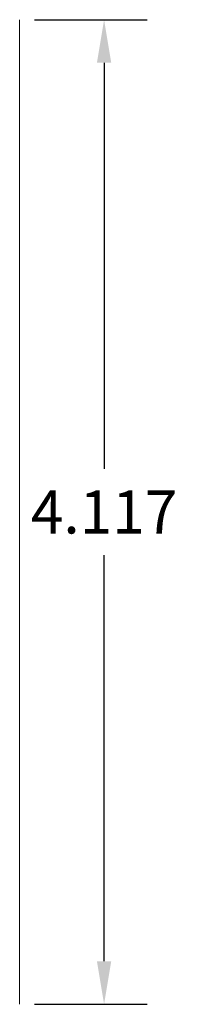
# Model space of a CAD drawing. Units: inches. Extents: x 0 to 0.66, y 7.93 to 12.04.
import ezdxf

# ---------------------------------------------------------------- set-up
doc = ezdxf.new("R2010")
doc.units = ezdxf.units.IN
doc.header["$MEASUREMENT"] = 0
doc.layers.add('M-CONS', color=7, linetype='Continuous', lineweight=18)
doc.layers.add('M-DIMS', color=2, linetype='Continuous', lineweight=18)
doc.styles.get("Standard").update_dxf_attribs({"font": 'arial.ttf'})
doc.dimstyles.get("Standard").update_dxf_attribs({"dimtxt": 0.18, "dimasz": 0.18, "dimexe": 0.18, "dimexo": 0.0625, "dimgap": 0.09, "dimtad": 0, "dimtih": 1, "dimtoh": 1, "dimdec": 4, "dimzin": 0, "dimdsep": 46, "dimtxsty": 'Standard', "dimcen": 0.09, "dimadec": 0, "dimazin": 0, "dimtfac": 1, "dimtdec": 4, "dimtofl": 0, "dimtmove": 0, "dimatfit": 3, "dimfxl": 1, "dimtolj": 1, "dimtzin": 0, "dimarcsym": 0})

# ---------------------------------------------------------------- blocks, each defined once
blk = doc.blocks.new('*D1')
at = {"layer": 'Defpoints', "color": 0, "transparency": 16777216}
for p in [(0, 12.0447), (0.3535, 12.0447), (0, 7.9273)]:
    blk.add_point(p, dxfattribs=at)
at = {"layer": 'M-DIMS', "color": 0, "lineweight": -2, "transparency": 16777216}
for p, q in [((0.0625, 12.0447), (0.5335, 12.0447)), ((0.3535, 11.8647), (0.3535, 10.1664)), ((0.3535, 8.1073), (0.3535, 9.8056)), ((0.0625, 7.9273), (0.5335, 7.9273))]:
    blk.add_line(p, q, dxfattribs=at)
at = {"layer": 'M-DIMS', "color": 0, "transparency": 16777216}
for points in [[(0.3235, 11.8647), (0.3835, 11.8647), (0.3535, 12.0447)], [(0.3235, 8.1073), (0.3835, 8.1073), (0.3535, 7.9273)]]:
    blk.add_solid(points, dxfattribs=at)
at = {"layer": 'M-DIMS', "color": 0, "transparency": 16777216, "insert": (0.3535, 9.986), "char_height": 0.18, "attachment_point": 5}
blk.add_mtext('\\A1;4.117', dxfattribs=at)

msp = doc.modelspace()

# ---------------------------------------------------------------- linework, layer by layer
at = {"layer": 'M-CONS', "extrusion": (-1, 0, 0)}
msp.add_lwpolyline([(-12.0447, 26.6429), (-7.9273, 26.6429), (-7.9273, 22.887), (-12.0447, 22.887)], close=True, dxfattribs=at)

# ---------------------------------------------------------------- dimensions: what is measured, and where the dimension line sits
at = {"layer": 'M-DIMS'}
dim = msp.add_linear_dim(base=(0.3535, 12.0447), p1=(0, 7.9273), p2=(0, 12.0447), angle=90, dimstyle='Standard', override={"dimdec": 3, "dimlfac": 1, "dimrnd": 0, "dimzin": 0, "dimdsep": 46, "dimlunit": 2}, dxfattribs=at)
dim.commit()
dim.dimension.update_dxf_attribs({"geometry": '*D1', "text_midpoint": (0.3535, 9.986)})

doc.saveas('drawing.dxf')
